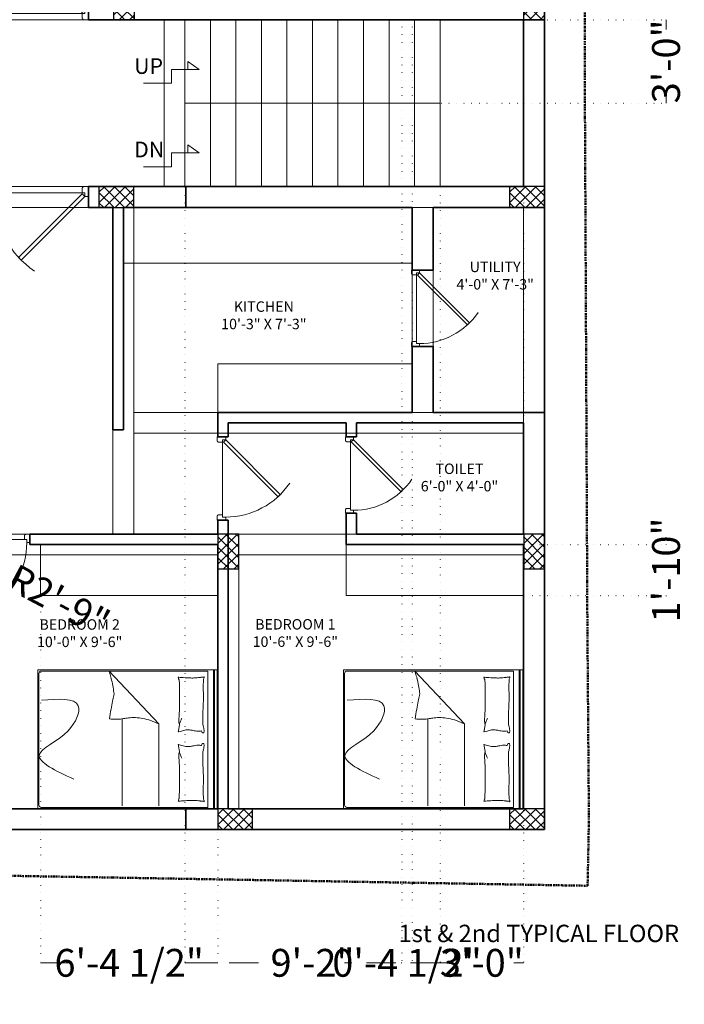
# Model space of a CAD drawing. Units: inches. Extents: x -16911 to -9621, y -48626 to -46270.
# Tile 7 of 20: x -11965 to -11679, y -48292 to -47867. Entities that reach past the tile are written whole.
import ezdxf

# ---------------------------------------------------------------- set-up
doc = ezdxf.new("R2010")
doc.units = ezdxf.units.IN
for name, pattern in [('DASHDOT', [1, 0.5, -0.25, 0, -0.25]), ('DASHED', [19.05, 12.7, -6.35]), ('DOT2', [3.175, 0, -3.175])]:
    doc.linetypes.add(name, pattern=pattern)
for name, color, linetype, lineweight in [('A-ANNO-DIMS', 2, 'Continuous', 13), ('A-ANNO-SYMB', 3, 'Continuous', 13), ('A-ANNO-TEXT', 7, 'Continuous', 18), ('A-AREA-IDEN', 3, 'Continuous', 18), ('A-DOOR', 4, 'Continuous', 18), ('A-FLOR-STRS', 3, 'Continuous', 18), ('A-FURN', 8, 'Continuous', 13), ('A-WALL', 7, 'Continuous', 35), ('C-PROP', 6, 'DASHDOT', 50), ('column', 12, 'Continuous', 30), ('DOOR', 143, 'Continuous', 9), ('EXT BEAM', 132, 'Continuous', 13), ('furniture', 35, 'Continuous', 15), ('S-BEAM', 132, 'Continuous', 25), ('S-COLS', 1, 'Continuous', 30), ('STAIRCASE', 137, 'Continuous', 5)]:
    doc.layers.add(name, color=color, linetype=linetype, lineweight=lineweight)
doc.styles.get("Standard").update_dxf_attribs({"font": 'swissel.ttf'})
doc.styles.add('style9', font='swisscl.ttf', dxfattribs={"height": 12})
doc.dimstyles.new('Dim9', dxfattribs={"dimtxt": 10, "dimasz": 0.199219, "dimexe": 1, "dimexo": 0.5, "dimgap": 1, "dimtad": 0, "dimdec": 1, "dimzin": 0, "dimdsep": 46, "dimlunit": 4, "dimtxsty": 'style9', "dimblk": 'ARCHTICK', "dimcen": 0.09, "dimclrd": 256, "dimclrt": 256, "dimadec": 0, "dimazin": 0, "dimtfac": 1, "dimtdec": 1, "dimtix": 1, "dimtofl": 0, "dimtmove": 1, "dimatfit": 3, "dimfxl": 9, "dimtolj": 1, "dimtzin": 0, "dimlwd": -1, "dimarcsym": 0})

# ---------------------------------------------------------------- blocks, each defined once
blk = doc.blocks.new('hjuyuiuyk')
at = {"layer": 'furniture'}
for p, q in [((-19327.49, -39738.98), (-19327.49, -39737.31)), ((-19327.49, -39737.31), (-19267.49, -39737.31, 0)), ((-19327.49, -39746.54), (-19327.49, -39737.31)), ((-19267.49, -39737.31, 0), (-19267.49, -39738.98, 0)), ((-19267.49, -39746.54, 0), (-19267.49, -39737.31, 0)), ((-19267.49, -39738.5), (-19327.49, -39738.5, 0)), ((-19327.49, -39738.5, 0), (-19327.49, -39814.72, 0)), ((-19327.49, -39738.5), (-19327.49, -39814.72)), ((-19267.49, -39738.5, 0), (-19327.49, -39738.5)), ((-19267.49, -39738.98, 0), (-19327.49, -39738.98)), ((-19268.1, -39741.33), (-19326.9, -39741.33)), ((-19326.9, -39741.33), (-19326.9, -39813.21)), ((-19268.1, -39813.21), (-19268.1, -39741.33)), ((-19267.49, -39814.72), (-19267.49, -39738.5)), ((-19267.49, -39814.72, 0), (-19267.49, -39738.5, 0)), ((-19300.88, -39753.22, 0), (-19301.49, -39750.81, 0)), ((-19300.67, -39754.09, 0), (-19300.88, -39753.22, 0)), ((-19295.19, -39754.09, 0), (-19294.97, -39753.22, 0)), ((-19294.97, -39753.22, 0), (-19294.37, -39750.81, 0)), ((-19304.07, -39762.52), (-19326.9, -39783.91)), ((-19304.07, -39762.52), (-19268.82, -39762.52)), ((-19268.82, -39778.34), (-19306.29, -39778.34)), ((-19326.9, -39813.21), (-19326.9, -39783.91)), ((-19269.1, -39814.21), (-19325.9, -39814.21)), ((-19325.9, -39814.21), (-19269.1, -39814.21)), ((-19327.49, -39814.72, 0), (-19267.49, -39814.72)), ((-19327.49, -39814.72), (-19267.49, -39814.72, 0))]:
    blk.add_line(p, q, dxfattribs=at)
for centre, radius, start, end in [((-19324.36, -39743.07, 0), 0.0997, 111.7883, 160.436), ((-19324.39, -39743.06, 0), 0.0676, 160.436, 281.8931), ((-19324.12, -39743.66, 0), 0.732, 94.3025, 111.7883), ((-19324.35, -39743.25, 0), 0.125, 21.9904, 101.8931), ((-19323.34, -39743.89, 0), 0.956, 158.579, 188.1335), ((-19317.18, -39743.01, 0), 7.17, 188.1335, 192.1095), ((-19324.65, -39743.37, 0), 0.455, 338.579, 21.9904), ((-19329.85, -39745.73, 0), 5.78, 7.6809, 12.1095), ((-19324.11, -39743.77, 0), 0.842, 59.3487, 94.3025), ((-19350.51, -39748.51, 0), 26.62, 3.3687, 7.6809), ((-19322.88, -39741.69, 0), 1.57, 239.3487, 264.7408), ((-19319.6, -39692.5, 0), 50.87, 266.1399, 268.6002), ((-19319.84, -39713.09, 0), 30.28, 268.0921, 271.2808), ((-19320.24, -39695.07, 0), 48.31, 271.2808, 273.4034), ((-19316.15, -39763.89, 0), 20.63, 90.1553, 93.4034), ((-19316.09, -39783.15, 0), 39.89, 86.9902, 90.1553), ((-19305.86, -39588.51, 0), 155.02, 266.9902, 268.5957), ((-19305.42, -39570.46, 0), 173.07, 268.5957, 270), ((-19305.42, -39718.38, 0), 25.15, 270, 273.6841), ((-19304.03, -39739.9, 0), 3.58, 273.6841, 287.1951), ((-19300.46, -39751.46, 0), 8.51, 98.4372, 107.1951), ((-19301.02, -39747.69, 0), 4.7, 90, 98.4372), ((-19301.12, -39743.14, 0), 0.997, 274.4002, 333.4195), ((-19315.3, -39745.68, 0), 14.34, 360, 6.2324), ((-19306.91, -39745.68, 0), 5.95, 350.3156, 360), ((-19301.02, -39745.63, 0), 2.64, 78.7276, 90), ((-19300.58, -39743.42, 0), 0.383, 333.4195, 78.7276), ((-19295.28, -39743.42, 0), 0.383, 101.2724, 206.5805), ((-19294.73, -39743.14, 0), 0.997, 206.5805, 265.5998), ((-19294.84, -39745.63, 0), 2.64, 90, 101.2724), ((-19280.55, -39745.68, 0), 14.34, 173.7676, 180), ((-19288.94, -39745.68, 0), 5.95, 180, 189.6844), ((-19294.84, -39747.69, 0), 4.7, 81.5628, 90), ((-19295.39, -39751.46, 0), 8.51, 72.8049, 81.5628), ((-19291.82, -39739.9, 0), 3.58, 252.8049, 266.3159), ((-19290.43, -39718.38, 0), 25.15, 266.3159, 270), ((-19290.43, -39570.46, 0), 173.07, 270, 271.4043), ((-19289.99, -39588.51, 0), 155.02, 271.4043, 273.0098), ((-19279.76, -39783.15, 0), 39.89, 89.8447, 93.0098), ((-19279.7, -39763.89, 0), 20.63, 86.5966, 89.8447), ((-19275.61, -39695.07, 0), 48.31, 266.5966, 268.7192), ((-19276.02, -39713.09, 0), 30.28, 268.7192, 271.9079), ((-19276.73, -39645.13, 0), 98.25, 271.0069, 272.7772), ((-19272.12, -39741.69, 0), 1.57, 275.2592, 300.6513), ((-19270.89, -39743.77, 0), 0.842, 85.6975, 120.6513), ((-19244.49, -39748.51, 0), 26.62, 172.3191, 176.6313), ((-19265.15, -39745.73, 0), 5.78, 167.8905, 172.3191), ((-19270.88, -39743.66, 0), 0.732, 68.2117, 85.6975), ((-19270.35, -39743.37, 0), 0.455, 158.0096, 201.421), ((-19277.82, -39743.01, 0), 7.17, 347.8905, 351.8665), ((-19270.65, -39743.25, 0), 0.125, 78.1069, 158.0096), ((-19271.66, -39743.89, 0), 0.956, 351.8665, 21.421), ((-19270.61, -39743.06, 0), 0.0676, 258.1069, 19.564), ((-19270.64, -39743.07, 0), 0.0997, 19.564, 68.2117), ((-19720.99, -39728.47, 0), 397.61, 356.4951, 356.945), ((-19363.7, -39747.54, 0), 39.81, 356.945, 358.3669), ((-19343.69, -39748.11, 0), 19.79, 358.3669, 3.3687), ((-19299.57, -39750.33, 0), 1.97, 177.3351, 194.0452), ((-19282.35, -39751.13, 0), 19.21, 171.9949, 177.3351), ((-19292.22, -39749.75, 0), 9.25, 167.8016, 171.9949), ((-19326.4, -39742.36, 0), 25.72, 347.8016, 350.3156), ((-19269.45, -39742.36, 0), 25.72, 189.6844, 192.1984), ((-19303.63, -39749.75, 0), 9.25, 8.0051, 12.1984), ((-19313.5, -39751.13, 0), 19.21, 2.6649, 8.0051), ((-19296.28, -39750.33, 0), 1.97, 345.9548, 2.6649), ((-19251.31, -39748.11, 0), 19.79, 176.6313, 181.6331), ((-19231.3, -39747.54, 0), 39.81, 181.6331, 183.055), ((-18874.01, -39728.47, 0), 397.61, 183.055, 183.5049), ((-19323.69, -39753.93, 0), 0.564, 170.0016, 196.6978), ((-19333.47, -39752.21, 0), 9.37, 350.0016, 356.4951), ((-19324.19, -39754.08, 0), 0.0385, 196.6978, 277.1204), ((-19324.51, -39751.59, 0), 2.55, 277.1204, 286.2212), ((-19324.42, -39751.9, 0), 2.23, 286.2212, 297.4439), ((-19322.81, -39754.99, 0), 1.25, 102.448, 117.4439), ((-19322.32, -39757.22, 0), 3.54, 93.574, 102.448), ((-19318.44, -39837.61, 0), 84.03, 90.9755, 92.7955), ((-19315.55, -39952.16, 0), 198.61, 89.4461, 91.2473), ((-19314.9, -39885.06, 0), 131.51, 87.2326, 89.4461), ((-19310.57, -39795.48, 0), 41.81, 85.4012, 87.2326), ((-19304.32, -39717.78, 0), 36.14, 265.4012, 267.3712), ((-19297.32, -39733.09, 0), 21.54, 244.6889, 246.5156), ((-19305.66, -39747.05, 0), 6.83, 267.3712, 281.4827), ((-19297.32, -39733.09, 0), 21.54, 246.5156, 248.3423), ((-19297.32, -39733.09, 0), 21.54, 248.3423, 250.572), ((-19297.32, -39733.09, 0), 21.54, 250.572, 252.8018), ((-19303.46, -39757.91, 0), 4.25, 83.5659, 101.4827), ((-19303.37, -39757.16, 0), 3.49, 72.6136, 83.5659), ((-19300.33, -39747.43, 0), 6.7, 252.6136, 260.5159), ((-19300.13, -39746.25, 0), 7.9, 260.5159, 265.9171), ((-19300.69, -39754.1, 0), 0.0267, 265.9171, 14.0449), ((-19295.16, -39754.1, 0), 0.0267, 165.9551, 274.0829), ((-19295.72, -39746.25, 0), 7.9, 274.0829, 279.4841), ((-19295.52, -39747.43, 0), 6.7, 279.4841, 287.3864), ((-19292.48, -39757.16, 0), 3.49, 96.4341, 107.3864), ((-19292.39, -39757.91, 0), 4.25, 78.5173, 96.4341), ((-19298.54, -39733.09, 0), 21.54, 287.1982, 289.428), ((-19290.19, -39747.05, 0), 6.83, 258.5173, 272.6288), ((-19298.54, -39733.09, 0), 21.54, 289.428, 291.6577), ((-19298.54, -39733.09, 0), 21.54, 291.6577, 293.4844), ((-19298.54, -39733.09, 0), 21.54, 293.4844, 295.3111), ((-19291.53, -39717.78, 0), 36.14, 272.6288, 274.5988), ((-19285.28, -39795.48, 0), 41.81, 92.7674, 94.5988), ((-19280.95, -39885.06, 0), 131.51, 90.5539, 92.7674), ((-19280.3, -39952.16, 0), 198.61, 88.7527, 90.5539), ((-19277.1, -39805.01, 0), 51.42, 86.426, 88.7527), ((-19274.68, -39799.75, 0), 46.07, 86.5575, 89.0171), ((-19272.19, -39754.99, 0), 1.25, 62.5561, 77.552), ((-19270.58, -39751.9, 0), 2.23, 242.5561, 253.7788), ((-19270.49, -39751.59, 0), 2.55, 253.7788, 262.8796), ((-19261.53, -39752.21, 0), 9.37, 183.5049, 189.9984), ((-19270.81, -39754.08, 0), 0.0385, 262.8796, 343.3022), ((-19271.31, -39753.93, 0), 0.564, 343.3022, 9.9984), ((-19279.47, -39774.89), 27.53, 153.3084, 168.7423), ((-19287.94, -39773.2), 18.89, 168.7423, 187.3994), ((-19242.78, -39767.34), 64.43, 187.3994, 189.2719), ((-19333.07, -39782.08), 27.05, 6.3817, 9.2719), ((-19321.79, -39780.82), 15.7, 359.2313, 6.3817), ((-19306.77, -39846.83), 66.07, 105.9352, 107.7364), ((-19318.41, -39806.06), 23.67, 102.9255, 105.9352), ((-19287.64, -39956.87), 177.57, 99.7243, 101.7196), ((-19317.24, -39783.9), 2.09, 82.2696, 100.7276), ((-19317.9, -39788.76), 6.99, 76.8096, 82.2696), ((-19295.64, -39693.77), 90.57, 256.8096, 258.3259), ((-19295.11, -39691.23), 93.17, 258.3259, 260.505), ((-19288.03, -39648.9), 136.08, 260.505, 262.308), ((-19336.71, -39780.62), 30.63, 354.1141, 359.2313), ((-19325.9, -39813.21), 1, 180, 270), ((-19269.1, -39813.21), 1, 270, 0)]:
    blk.add_arc(centre, radius, start, end, dxfattribs=at)
blk.add_open_spline([(-19280.24, -39799.21), (-19283.87, -39806.94), (-19290.73, -39821.55), (-19298.08, -39801.09), (-19315.85, -39793.47), (-19314.86, -39805.92), (-19314.29, -39813.13)], degree=3, knots=[0, 0, 0, 0, 18.167809, 34.338432, 45.972904, 61.997799, 61.997799, 61.997799, 61.997799], dxfattribs=at)
blk = doc.blocks.new('A$C1C9D3E54')
at = {"layer": 'DOOR'}
blk.add_line((18676.53, 5780.72), (18710.53, 5780.72), dxfattribs=at)
blk.add_lwpolyline([(18685.01, 5806.62), (18710.47, 5781.16), (18711.53, 5782.22), (18686.07, 5807.68), (18685.01, 5806.62)], dxfattribs=at)
blk.add_lwpolyline([(18674.03, 5778.22), (18676.03, 5778.22), (18674.03, 5778.22), (18674.03, 5782.22), (18675.53, 5782.22), (18675.53, 5780.72), (18676.53, 5780.72), (18676.53, 5778.72), (18676.41, 5778.72), (18676.41, 5778.6, -0.414214), (18676.16, 5778.35), (18676.03, 5778.35), (18676.03, 5778.22)], format="xyb", dxfattribs=at)
blk.add_lwpolyline([(18713.03, 5782.22), (18711.53, 5782.22), (18711.53, 5780.72), (18710.53, 5780.72), (18710.53, 5778.72), (18710.66, 5778.72), (18710.66, 5778.6, 0.414214), (18710.91, 5778.35), (18711.03, 5778.35), (18711.03, 5778.22), (18713.03, 5778.22), (18711.03, 5778.22), (18713.03, 5778.22), (18713.03, 5782.22)], format="xyb", close=True, dxfattribs=at)
blk.add_arc((18711.53, 5782.22), 36, 124.0336, 180, dxfattribs=at)
blk = doc.blocks.new('THYHYTJ')
at = {"layer": 'STAIRCASE', "ltscale": 10}
for p, q in [((-7981.18, -46346.18), (-7984.62, -46351.1)), ((-7981.18, -46358.18), (-7981.18, -46346.18)), ((-7984.62, -46351.1), (-7981.18, -46351.1)), ((-7975.18, -46358.18), (-7981.18, -46358.18)), ((-7975.18, -46370.18), (-7975.18, -46358.18))]:
    blk.add_line(p, q, dxfattribs=at)
blk = doc.blocks.new('COLUMNS')
at = {"layer": 'column'}
h = blk.add_hatch(dxfattribs=at)
h.set_pattern_fill('ANSI37', color=256, angle=-720)
h.set_pattern_definition([(45, (21840.2088, -104675.1704), (-2.24506403, 2.24506403), []), (135, (21840.2088, -104675.1704), (-2.24506403, -2.24506403), [])])
h.paths.add_polyline_path([(-11924.72, -46595.36), (-11915.72, -46595.36), (-11915.72, -46580.36), (-11924.72, -46580.36)])
h = blk.add_hatch(dxfattribs=at)
h.set_pattern_fill('ANSI37', color=256, angle=-900)
h.set_pattern_definition([(225, (-45503.8578, 11499.4594), (2.24506403, -2.24506403), []), (315, (-45503.8578, 11499.4594), (2.24506403, 2.24506403), [])])
h.paths.add_polyline_path([(-11738.92, -46580.36), (-11747.92, -46580.36), (-11747.92, -46595.36), (-11738.92, -46595.36)])
h = blk.add_hatch(dxfattribs=at)
h.set_pattern_fill('ANSI37', color=256, angle=-810)
h.set_pattern_definition([(315, (-70010.7892, -80432.2886), (2.24506403, 2.24506403), []), (45, (-70010.7892, -80432.2886), (-2.24506403, 2.24506403), [])])
h.paths.add_polyline_path([(-11930.97, -46667.36), (-11930.97, -46676.36), (-11915.97, -46676.36), (-11915.97, -46667.36)])
h = blk.add_hatch(dxfattribs=at)
h.set_pattern_fill('ANSI37', color=256, angle=-810)
h.set_pattern_definition([(315, (-69833.7395, -80432.2886), (2.24506403, 2.24506403), []), (45, (-69833.7395, -80432.2886), (-2.24506403, 2.24506403), [])])
h.paths.add_polyline_path([(-11753.92, -46667.36), (-11753.92, -46676.36), (-11738.92, -46676.36), (-11738.92, -46667.36)])
h = blk.add_hatch(dxfattribs=at)
h.set_pattern_fill('ANSI37', color=256, angle=-720)
h.set_pattern_definition([(45, (21885.2088, -104912.1242), (-2.24506403, 2.24506403), []), (135, (21885.2088, -104912.1242), (-2.24506403, -2.24506403), [])])
h.paths.add_polyline_path([(-11879.72, -46832.31), (-11870.72, -46832.31), (-11870.72, -46817.31), (-11879.72, -46817.31)])
h = blk.add_hatch(dxfattribs=at)
h.set_pattern_fill('ANSI37', color=256, angle=-720)
h.set_pattern_definition([(45, (22017.1023, -104912.1242), (-2.24506403, 2.24506403), []), (135, (22017.1023, -104912.1242), (-2.24506403, -2.24506403), [])])
h.paths.add_polyline_path([(-11747.83, -46832.31), (-11738.83, -46832.31), (-11738.83, -46817.31), (-11747.83, -46817.31)])
h = blk.add_hatch(dxfattribs=at)
h.set_pattern_fill('ANSI37', color=256, angle=-810)
h.set_pattern_definition([(315, (-69959.5392, -80700.7425), (2.24506403, 2.24506403), []), (45, (-69959.5392, -80700.7425), (-2.24506403, 2.24506403), [])])
h.paths.add_polyline_path([(-11879.72, -46935.81), (-11879.72, -46944.81), (-11864.72, -46944.81), (-11864.72, -46935.81)])
h = blk.add_hatch(dxfattribs=at)
h.set_pattern_fill('ANSI37', color=256, angle=-810)
h.set_pattern_definition([(315, (-69833.7395, -80700.7425), (2.24506403, 2.24506403), []), (45, (-69833.7395, -80700.7425), (-2.24506403, 2.24506403), [])])
h.paths.add_polyline_path([(-11753.92, -46935.81), (-11753.92, -46944.81), (-11738.92, -46944.81), (-11738.92, -46935.81)])
at = {"layer": 'column', "ltscale": 0.05}
for points in [[(-11915.72, -46580.36), (-11924.72, -46580.36), (-11924.72, -46595.36), (-11915.72, -46595.36)], [(-11747.92, -46595.36), (-11738.92, -46595.36), (-11738.92, -46580.36), (-11747.92, -46580.36)], [(-11915.97, -46676.36), (-11915.97, -46667.36), (-11930.97, -46667.36), (-11930.97, -46676.36)], [(-11738.92, -46676.36), (-11738.92, -46667.36), (-11753.92, -46667.36), (-11753.92, -46676.36)], [(-11870.72, -46817.31), (-11879.72, -46817.31), (-11879.72, -46832.31), (-11870.72, -46832.31)], [(-11738.83, -46817.31), (-11747.83, -46817.31), (-11747.83, -46832.31), (-11738.83, -46832.31)], [(-11864.72, -46944.81), (-11864.72, -46935.81), (-11879.72, -46935.81), (-11879.72, -46944.81)], [(-11738.92, -46944.81), (-11738.92, -46935.81), (-11753.92, -46935.81), (-11753.92, -46944.81)]]:
    blk.add_lwpolyline(points, close=True, dxfattribs=at)
blk = doc.blocks.new('TYPICAL BEAMS G-2')
at = {"layer": 'EXT BEAM'}
for p, q in [((-11738.92, -48216.7), (-11738.92, -47658.74)), ((-12052.47, -47867.24), (-11924.72, -47867.24)), ((-11915.72, -47867.24), (-11747.92, -47867.24)), ((-11902.92, -47867.24), (-11902.92, -47939.24)), ((-11893.92, -47867.24), (-11893.92, -47939.24)), ((-11747.92, -47939.24), (-11747.92, -47867.24)), ((-12046.47, -47939.24), (-11929.47, -47939.24)), ((-11920.47, -47939.24), (-11738.92, -47939.24)), ((-12046.47, -47948.24), (-11929.47, -47948.24)), ((-11924.97, -47948.24), (-11924.97, -48089.2)), ((-11920.47, -47948.24), (-11738.92, -47948.24)), ((-11915.97, -47948.24), (-11915.97, -48089.2)), ((-11795.92, -47948.24), (-11795.92, -48036.7)), ((-11786.92, -47948.24), (-11786.92, -48036.7)), ((-11747.92, -48089.2), (-11747.92, -47948.24)), ((-11747.92, -48036.7), (-11915.97, -48036.7)), ((-11747.92, -48045.7), (-11915.97, -48045.7)), ((-12052.47, -48089.2), (-11747.92, -48089.2)), ((-12052.47, -48098.2), (-11879.72, -48098.2)), ((-11879.72, -48098.2), (-11879.72, -48207.7)), ((-11870.72, -48098.2), (-11747.92, -48098.2)), ((-11870.72, -48098.2), (-11870.72, -48207.7)), ((-11747.92, -48207.7), (-11747.92, -48098.2)), ((-12052.47, -48207.7), (-11879.72, -48207.7)), ((-11870.72, -48207.7), (-11747.92, -48207.7)), ((-12061.47, -48216.7), (-11738.92, -48216.7))]:
    blk.add_line(p, q, dxfattribs=at)
blk = doc.blocks.new('_ArchTick')
at = {"color": 0, "linetype": 'ByBlock', "const_width": 0.15}
blk.add_lwpolyline([(-0.5, -0.5), (0.5, 0.5)], dxfattribs=at)
blk = doc.blocks.new('*D117')
at = {"layer": 'A-ANNO-DIMS', "color": 0, "linetype": 'DOT2', "lineweight": -2, "transparency": 16777216}
for p, q in [((-11893.92, -47939.74), (-11893.92, -48275.17)), ((-11783.92, -47939.74), (-11783.92, -48275.17))]:
    blk.add_line(p, q, dxfattribs=at)
at = {"layer": 'A-ANNO-DIMS', "linetype": 'DASHED', "transparency": 16777216}
for p, q in [((-11893.92, -48274.17), (-11852.75, -48274.17)), ((-11783.92, -48274.17), (-11825.1, -48274.17))]:
    blk.add_line(p, q, dxfattribs=at)
at = {"layer": 'Defpoints', "color": 0, "transparency": 16777216}
for p in [(-11893.92, -47939.24), (-11783.92, -47939.24), (-11783.92, -48274.17)]:
    blk.add_point(p, dxfattribs=at)
at = {"layer": 'A-ANNO-DIMS', "transparency": 16777216, "xscale": 0.19921875, "yscale": 0.19921875, "zscale": 0.19921875, "rotation": 180}
blk.add_blockref('_ArchTick', (-11893.92, -48274.17), dxfattribs=at)
at = {"layer": 'A-ANNO-DIMS', "transparency": 16777216, "xscale": 0.19921875, "yscale": 0.19921875, "zscale": 0.19921875}
blk.add_blockref('_ArchTick', (-11783.92, -48274.17), dxfattribs=at)
at = {"layer": 'A-ANNO-DIMS', "transparency": 16777216, "insert": (-11838.92, -48274.17), "char_height": 12, "attachment_point": 5, "style": 'style9'}
blk.add_mtext('\\A1;9\'-2"', dxfattribs=at)
blk = doc.blocks.new('*D118')
at = {"layer": 'A-ANNO-DIMS', "color": 0, "linetype": 'DOT2', "lineweight": -2, "transparency": 16777216}
for p, q in [((-11783.92, -47939.74), (-11783.92, -48275.17)), ((-11747.92, -47939.74), (-11747.92, -48275.17))]:
    blk.add_line(p, q, dxfattribs=at)
at = {"layer": 'A-ANNO-DIMS', "linetype": 'DASHED', "transparency": 16777216}
for p, q in [((-11783.92, -48274.17), (-11779.73, -48274.17)), ((-11747.92, -48274.17), (-11752.12, -48274.17))]:
    blk.add_line(p, q, dxfattribs=at)
at = {"layer": 'Defpoints', "color": 0, "transparency": 16777216}
for p in [(-11783.92, -47939.24), (-11747.92, -47939.24), (-11747.92, -48274.17)]:
    blk.add_point(p, dxfattribs=at)
at = {"layer": 'A-ANNO-DIMS', "transparency": 16777216, "xscale": 0.19921875, "yscale": 0.19921875, "zscale": 0.19921875, "rotation": 180}
blk.add_blockref('_ArchTick', (-11783.92, -48274.17), dxfattribs=at)
at = {"layer": 'A-ANNO-DIMS', "transparency": 16777216, "xscale": 0.19921875, "yscale": 0.19921875, "zscale": 0.19921875}
blk.add_blockref('_ArchTick', (-11747.92, -48274.17), dxfattribs=at)
at = {"layer": 'A-ANNO-DIMS', "transparency": 16777216, "insert": (-11765.92, -48274.17), "char_height": 12, "attachment_point": 5, "style": 'style9'}
blk.add_mtext('\\A1;3\'-0"', dxfattribs=at)
blk = doc.blocks.new('*D119')
at = {"layer": 'A-ANNO-DIMS', "color": 0, "linetype": 'DOT2', "lineweight": -2, "transparency": 16777216}
for p, q in [((-11783.42, -47867.24), (-11685.48, -47867.24)), ((-11783.42, -47903.24), (-11685.48, -47903.24))]:
    blk.add_line(p, q, dxfattribs=at)
at = {"layer": 'A-ANNO-DIMS', "linetype": 'DASHED', "transparency": 16777216}
for p, q in [((-11686.48, -47867.24), (-11686.48, -47871.44)), ((-11686.48, -47903.24), (-11686.48, -47899.05))]:
    blk.add_line(p, q, dxfattribs=at)
at = {"layer": 'Defpoints', "color": 0, "transparency": 16777216}
for p in [(-11783.92, -47867.24), (-11783.92, -47903.24), (-11686.48, -47903.24)]:
    blk.add_point(p, dxfattribs=at)
at = {"layer": 'A-ANNO-DIMS', "transparency": 16777216, "xscale": 0.19921875, "yscale": 0.19921875, "zscale": 0.19921875}
for p, rotation in [((-11686.48, -47867.24), 90), ((-11686.48, -47903.24), 270)]:
    blk.add_blockref('_ArchTick', p, dxfattribs=dict(at, rotation=rotation))
at = {"layer": 'A-ANNO-DIMS', "transparency": 16777216, "insert": (-11686.48, -47885.24), "char_height": 12, "attachment_point": 5, "rotation": 90, "style": 'style9'}
blk.add_mtext('\\A1;3\'-0"', dxfattribs=at)
blk = doc.blocks.new('*D120')
at = {"layer": 'A-ANNO-DIMS', "color": 0, "linetype": 'DOT2', "lineweight": -2, "transparency": 16777216}
for p, q in [((-11747.42, -48093.7), (-11685.48, -48093.7)), ((-11747.42, -48115.7), (-11685.48, -48115.7))]:
    blk.add_line(p, q, dxfattribs=at)
at = {"layer": 'A-ANNO-DIMS', "linetype": 'DASHED', "transparency": 16777216}
for p, q in [((-11686.48, -48093.7), (-11686.48, -48093.5)), ((-11686.48, -48115.7), (-11686.48, -48115.9))]:
    blk.add_line(p, q, dxfattribs=at)
at = {"layer": 'Defpoints', "color": 0, "transparency": 16777216}
for p in [(-11747.92, -48093.7), (-11747.92, -48115.7), (-11686.48, -48115.7)]:
    blk.add_point(p, dxfattribs=at)
at = {"layer": 'A-ANNO-DIMS', "transparency": 16777216, "xscale": 0.19921875, "yscale": 0.19921875, "zscale": 0.19921875}
for p, rotation in [((-11686.48, -48093.7), 270), ((-11686.48, -48115.7), 90)]:
    blk.add_blockref('_ArchTick', p, dxfattribs=dict(at, rotation=rotation))
at = {"layer": 'A-ANNO-DIMS', "transparency": 16777216, "insert": (-11686.48, -48104.7), "char_height": 12, "attachment_point": 5, "rotation": 90, "style": 'style9'}
blk.add_mtext('\\A1;1\'-10"', dxfattribs=at)
blk = doc.blocks.new('*D121')
at = {"layer": 'A-ANNO-DIMS', "color": 0, "linetype": 'DOT2', "lineweight": -2, "transparency": 16777216}
for p, q in [((-11956.22, -48116.2), (-11956.22, -48275.17)), ((-11879.72, -48116.2), (-11879.72, -48275.17))]:
    blk.add_line(p, q, dxfattribs=at)
at = {"layer": 'A-ANNO-DIMS', "linetype": 'DASHED', "transparency": 16777216}
for p, q in [((-11956.22, -48274.17), (-11943.49, -48274.17)), ((-11879.72, -48274.17), (-11892.46, -48274.17))]:
    blk.add_line(p, q, dxfattribs=at)
at = {"layer": 'Defpoints', "color": 0, "transparency": 16777216}
for p in [(-11956.22, -48115.7), (-11879.72, -48115.7), (-11879.72, -48274.17)]:
    blk.add_point(p, dxfattribs=at)
at = {"layer": 'A-ANNO-DIMS', "transparency": 16777216, "xscale": 0.19921875, "yscale": 0.19921875, "zscale": 0.19921875, "rotation": 180}
blk.add_blockref('_ArchTick', (-11956.22, -48274.17), dxfattribs=at)
at = {"layer": 'A-ANNO-DIMS', "transparency": 16777216, "xscale": 0.19921875, "yscale": 0.19921875, "zscale": 0.19921875}
blk.add_blockref('_ArchTick', (-11879.72, -48274.17), dxfattribs=at)
at = {"layer": 'A-ANNO-DIMS', "transparency": 16777216, "insert": (-11917.97, -48274.17), "char_height": 12, "attachment_point": 5, "style": 'style9'}
blk.add_mtext('\\A1;6\'-4 1/2"', dxfattribs=at)
blk = doc.blocks.new('*D122')
at = {"layer": 'A-ANNO-DIMS', "color": 0, "linetype": 'DOT2', "lineweight": -2, "transparency": 16777216}
for p, q in [((-11800.42, -47821.24), (-11800.42, -48275.17)), ((-11795.92, -47821.24), (-11795.92, -48275.17))]:
    blk.add_line(p, q, dxfattribs=at)
at = {"layer": 'A-ANNO-DIMS', "linetype": 'DASHED', "transparency": 16777216}
for p, q in [((-11800.42, -48274.17), (-11800.62, -48274.17)), ((-11795.92, -48274.17), (-11795.73, -48274.17))]:
    blk.add_line(p, q, dxfattribs=at)
at = {"layer": 'Defpoints', "color": 0, "transparency": 16777216}
for p in [(-11800.42, -47820.74), (-11795.92, -47820.74), (-11795.92, -48274.17)]:
    blk.add_point(p, dxfattribs=at)
at = {"layer": 'A-ANNO-DIMS', "transparency": 16777216, "xscale": 0.19921875, "yscale": 0.19921875, "zscale": 0.19921875}
blk.add_blockref('_ArchTick', (-11800.42, -48274.17), dxfattribs=at)
at = {"layer": 'A-ANNO-DIMS', "transparency": 16777216, "xscale": 0.19921875, "yscale": 0.19921875, "zscale": 0.19921875, "rotation": 180}
blk.add_blockref('_ArchTick', (-11795.92, -48274.17), dxfattribs=at)
at = {"layer": 'A-ANNO-DIMS', "transparency": 16777216, "insert": (-11798.17, -48274.17), "char_height": 12, "attachment_point": 5, "style": 'style9'}
blk.add_mtext('\\A1;0\'-4 1/2"', dxfattribs=at)
blk = doc.blocks.new('*D136')
at = {"layer": 'A-ANNO-DIMS', "color": 0, "lineweight": -2, "transparency": 16777216}
for p, q in [((-11995.43, -48092.88), (-11995.25, -48092.88)), ((-11995.34, -48092.97), (-11995.34, -48092.79))]:
    blk.add_line(p, q, dxfattribs=at)
at = {"layer": 'A-ANNO-DIMS', "linetype": 'DASHED', "transparency": 16777216}
blk.add_line((-11964.07, -48109.5), (-11965.99, -48108.48), dxfattribs=at)
at = {"layer": 'Defpoints', "color": 0, "transparency": 16777216}
for p in [(-11995.34, -48092.88), (-11965.99, -48108.48)]:
    blk.add_point(p, dxfattribs=at)
at = {"layer": 'A-ANNO-DIMS', "transparency": 16777216, "xscale": 0.19921875, "yscale": 0.19921875, "zscale": 0.19921875, "rotation": 152.0167210822722}
blk.add_blockref('_ArchTick', (-11965.99, -48108.48), dxfattribs=at)
at = {"layer": 'A-ANNO-DIMS', "transparency": 16777216, "insert": (-11948.39, -48117.83), "char_height": 12, "attachment_point": 5, "rotation": 332.0167, "style": 'style9'}
blk.add_mtext('\\A1;R2\'-9"', dxfattribs=at)

msp = doc.modelspace()

# ---------------------------------------------------------------- linework, layer by layer
at = {"layer": 'A-FLOR-STRS', "ltscale": 10}
for p, q in [((-11893.925, -47867.242), (-11893.925, -47939.242)), ((-11882.925, -47867.242), (-11882.925, -47939.242)), ((-11871.925, -47867.242), (-11871.925, -47939.242)), ((-11860.925, -47867.242), (-11860.925, -47939.242)), ((-11849.925, -47867.242), (-11849.925, -47939.242)), ((-11838.925, -47867.242), (-11838.925, -47939.242)), ((-11827.925, -47867.242), (-11827.925, -47939.242)), ((-11816.925, -47867.242), (-11816.925, -47939.242)), ((-11805.925, -47867.242), (-11805.925, -47939.242)), ((-11794.925, -47867.242), (-11794.925, -47939.242)), ((-11783.925, -47867.242), (-11783.925, -47939.242)), ((-11783.925, -47903.242), (-11893.925, -47903.242))]:
    msp.add_line(p, q, dxfattribs=at)
at = {"layer": 'A-FURN', "ltscale": 0.2}
for p, q in [((-11795.925, -47972.242), (-11920.474, -47972.242)), ((-11795.925, -48015.696), (-11879.724, -48015.696)), ((-11879.724, -48036.696), (-11879.724, -48015.696)), ((-11956.224, -48093.696, 0), (-11956.224, -48115.696, 0)), ((-11824.425, -48093.696), (-11824.425, -48115.696)), ((-11879.724, -48115.696), (-11956.224, -48115.696)), ((-11824.425, -48115.696), (-11747.925, -48115.696))]:
    msp.add_line(p, q, dxfattribs=at)
at = {"layer": 'A-WALL'}
for p, q in [((-11738.925, -47741.242), (-11738.925, -47948.242)), ((-11935.474, -47867.242), (-11935.474, -47858.242)), ((-11738.925, -47858.242), (-11738.925, -47867.242)), ((-11738.925, -47867.242), (-11935.474, -47867.242)), ((-11747.925, -47867.242), (-11747.925, -47939.242)), ((-11747.925, -47939.242), (-11935.474, -47939.242)), ((-11935.474, -47948.242), (-11935.474, -47939.242)), ((-11893.506, -47939.242), (-11893.506, -47948.242)), ((-11738.925, -47939.242), (-11738.925, -47948.242)), ((-11924.974, -47948.242), (-11935.474, -47948.242)), ((-11924.974, -47948.242), (-11924.974, -48044.242)), ((-11795.925, -47948.242), (-11920.474, -47948.242)), ((-11920.474, -47948.242), (-11920.474, -48044.242)), ((-11795.925, -47948.242), (-11795.925, -47975.242)), ((-11738.925, -47948.242), (-11786.925, -47948.242)), ((-11786.925, -47948.242), (-11786.925, -47975.242)), ((-11738.925, -47948.242), (-11738.925, -48036.696)), ((-11795.925, -47975.242), (-11786.925, -47975.242)), ((-11795.925, -48008.242), (-11795.925, -48036.696)), ((-11795.925, -48008.242), (-11786.925, -48008.242)), ((-11786.925, -48008.242), (-11786.925, -48036.696)), ((-11879.724, -48047.196), (-11879.724, -48036.696)), ((-11879.724, -48036.696), (-11795.925, -48036.696)), ((-11786.925, -48036.696), (-11738.925, -48036.696)), ((-11738.925, -48036.696), (-11738.925, -48216.696)), ((-11875.224, -48047.196), (-11875.224, -48041.196)), ((-11875.224, -48041.196), (-11824.425, -48041.196)), ((-11824.425, -48041.196), (-11824.425, -48047.196)), ((-11819.925, -48041.196), (-11819.925, -48047.196)), ((-11819.925, -48041.196), (-11747.925, -48041.196)), ((-11747.925, -48041.196), (-11747.925, -48089.196)), ((-11920.474, -48044.242), (-11924.974, -48044.242)), ((-11879.724, -48047.196), (-11875.224, -48047.196)), ((-11824.425, -48047.196), (-11819.925, -48047.196)), ((-11824.425, -48080.196), (-11824.425, -48093.696)), ((-11824.425, -48080.196), (-11819.925, -48080.196)), ((-11819.925, -48080.196), (-11819.925, -48089.196)), ((-11879.724, -48089.196), (-11879.724, -48083.196)), ((-11879.724, -48083.196), (-11875.224, -48083.196)), ((-11875.224, -48207.696), (-11875.224, -48083.196)), ((-11960.724, -48089.196), (-11879.724, -48089.196)), ((-11960.724, -48093.696), (-11960.724, -48089.196)), ((-11819.925, -48089.196), (-11747.925, -48089.196)), ((-11960.724, -48093.696), (-11879.724, -48093.696)), ((-11879.724, -48207.696), (-11879.724, -48093.696)), ((-11824.425, -48093.696), (-11747.925, -48093.696)), ((-11747.925, -48093.696), (-11747.925, -48207.696)), ((-11999.974, -48207.696), (-11879.724, -48207.696)), ((-11893.506, -48207.696), (-11893.506, -48216.696)), ((-11875.224, -48207.696), (-11747.925, -48207.696)), ((-11738.925, -48207.696), (-11738.925, -48216.696)), ((-12008.974, -48216.696), (-11738.925, -48216.696))]:
    msp.add_line(p, q, dxfattribs=at)
at = {"layer": 'C-PROP'}
msp.add_lwpolyline([(-12080.474, -48234.696), (-11720.293, -48240.921), (-11719.732, -48212.333), (-11720.395, -48127.492), (-11721.561, -47881.398), (-11721.175, -47639.742), (-12080.838, -47634.697), (-12080.3, -48034.841)], close=True, dxfattribs=at)

# ---------------------------------------------------------------- block references
at = {"layer": 'A-ANNO-SYMB', "rotation": 270.0000000000144}
for p in [(34458.429, -55869.844), (34458.429, -55905.844)]:
    msp.add_blockref('THYHYTJ', p, dxfattribs=at)
at = {"layer": 'A-DOOR', "xscale": 1.076923076922859, "yscale": 1.076923076922859, "zscale": 1.076923076922859}
msp.add_blockref('A$C1C9D3E54', (-32087.969, -54089.945), dxfattribs=at)
at = {"layer": 'A-DOOR'}
for p, xscale, yscale, zscale, rotation in [((-32087.969, -41716.539), -1.076923076922859, 1.076923076922859, 1.076923076922859, 180), ((-16685.441, -63809.345), -0.8461538461538624, 0.8461538461538624, 0.8461538461538624, 270), ((-17213.72, -65320.763), -0.9230769230769229, 0.9230769230769229, 0.9230769230769229, 270), ((-16713.941, -63881.299), -0.8461538461538624, 0.8461538461538624, 0.8461538461538624, 270), ((5276.842, -42755.451), 0.9230769230769229, 0.9230769230769229, 0.9230769230769229, 180)]:
    msp.add_blockref('A$C1C9D3E54', p, dxfattribs=dict(at, xscale=xscale, yscale=yscale, zscale=zscale, rotation=rotation))
at = {"layer": 'A-FURN', "rotation": 270}
for p in [(27857.338, -67475.182), (27989.137, -67475.182, 0)]:
    msp.add_blockref('hjuyuiuyk', p, dxfattribs=at)
at = {"layer": 'S-BEAM'}
msp.add_blockref('TYPICAL BEAMS G-2', (0, 0), dxfattribs=at)
at = {"layer": 'S-COLS'}
msp.add_blockref('COLUMNS', (0, -1271.886), dxfattribs=at)

# ---------------------------------------------------------------- texts
at = {"layer": 'A-ANNO-TEXT'}
for s, p in [('UP', (-11915.824, -47890.629)), ('DN', (-11915.824, -47926.629))]:
    msp.add_text(s, height=6.75, dxfattribs=at).set_placement(p)
at = {"layer": 'A-ANNO-TEXT', "ltscale": 10, "insert": (-11801.781, -48257.731), "char_height": 7.5, "width": 166.78033, "attachment_point": 1, "style": 'style9'}
msp.add_mtext('\\A1;{\\fCentury Gothic|b0|i0|c0|p34;1st & 2nd TYPICAL FLOOR}', dxfattribs=at)
at = {"layer": 'A-AREA-IDEN', "ltscale": 10, "char_height": 4.5, "width": 42.823, "attachment_point": 1, "style": 'style9'}
for s, insert in [('\\A1;\\pxqc;{\\fCentury Gothic|b0|i0|c0|p34;UTILITY\\P4\'-0" X 7\'-3"}', (-11781.564, -47971.658)), ('\\A1;\\pxqc;{\\fCentury Gothic|b0|i0|c0|p34;KITCHEN\\P10\'-3" X 7\'-3"}', (-11881.298, -47988.779)), ('\\A1;\\pxqc;{\\fCentury Gothic|b0|i0|c0|p34;TOILET\\P6\'-0" X 4\'-0"}', (-11796.951, -48058.76)), ('\\A1;\\pxqc;{\\fCentury Gothic|b0|i0|c0|p34;BEDROOM 2\\P10\'-0" X 9\'-6"}', (-11960.722, -48125.934)), ('\\A1;\\pxqc;{\\fCentury Gothic|b0|i0|c0|p34;BEDROOM 1\\P10\'-6" X 9\'-6"}', (-11867.728, -48125.858))]:
    msp.add_mtext(s, dxfattribs=dict(at, insert=insert))

# ---------------------------------------------------------------- dimensions: what is measured, and where the dimension line sits
at = {"layer": 'A-ANNO-DIMS'}
for base, p1, p2, picture, middle in [((-11795.925, -48274.171), (-11800.425, -47820.742), (-11795.925, -47820.742), '*D122', (-11798.175, -48274.171)), ((-11783.925, -48274.171), (-11893.925, -47939.242), (-11783.925, -47939.242), '*D117', (-11838.925, -48274.171)), ((-11747.925, -48274.171), (-11783.925, -47939.242), (-11747.925, -47939.242), '*D118', (-11765.925, -48274.171)), ((-11879.724, -48274.171), (-11956.224, -48115.696), (-11879.724, -48115.696), '*D121', (-11917.974, -48274.171))]:
    dim = msp.add_linear_dim(base=base, p1=p1, p2=p2, dimstyle='Dim9', override={"dimdec": 1, "dimlfac": 1, "dimrnd": 0, "dimzin": 1, "dimdsep": 46, "dimlunit": 4, "dimfrac": 2}, dxfattribs=at)
    dim.commit()
    dim.dimension.update_dxf_attribs({"geometry": picture, "text_midpoint": middle})
for base, p1, p2, picture, middle in [((-11686.482, -47903.242), (-11783.925, -47867.242), (-11783.925, -47903.242), '*D119', (-11686.482, -47885.242)), ((-11686.482, -48115.696), (-11747.925, -48093.696), (-11747.925, -48115.696), '*D120', (-11686.482, -48104.696))]:
    dim = msp.add_linear_dim(base=base, p1=p1, p2=p2, angle=90, dimstyle='Dim9', override={"dimdec": 1, "dimlfac": 1, "dimrnd": 0, "dimzin": 1, "dimdsep": 46, "dimlunit": 4, "dimfrac": 2}, dxfattribs=at)
    dim.commit()
    dim.dimension.update_dxf_attribs({"geometry": picture, "text_midpoint": middle})
dim = msp.add_radius_dim(center=(-11995.34, -48092.885), mpoint=(-11965.994, -48108.477), dimstyle='Dim9', override={"dimdec": 1, "dimlfac": 1, "dimrnd": 0, "dimzin": 1, "dimdsep": 46, "dimlunit": 4, "dimfrac": 2}, dxfattribs=at)
dim.commit()
dim.dimension.update_dxf_attribs({"geometry": '*D136', "text_midpoint": (-11948.387, -48117.832), "dimtype": 164})

doc.saveas('drawing.dxf')
